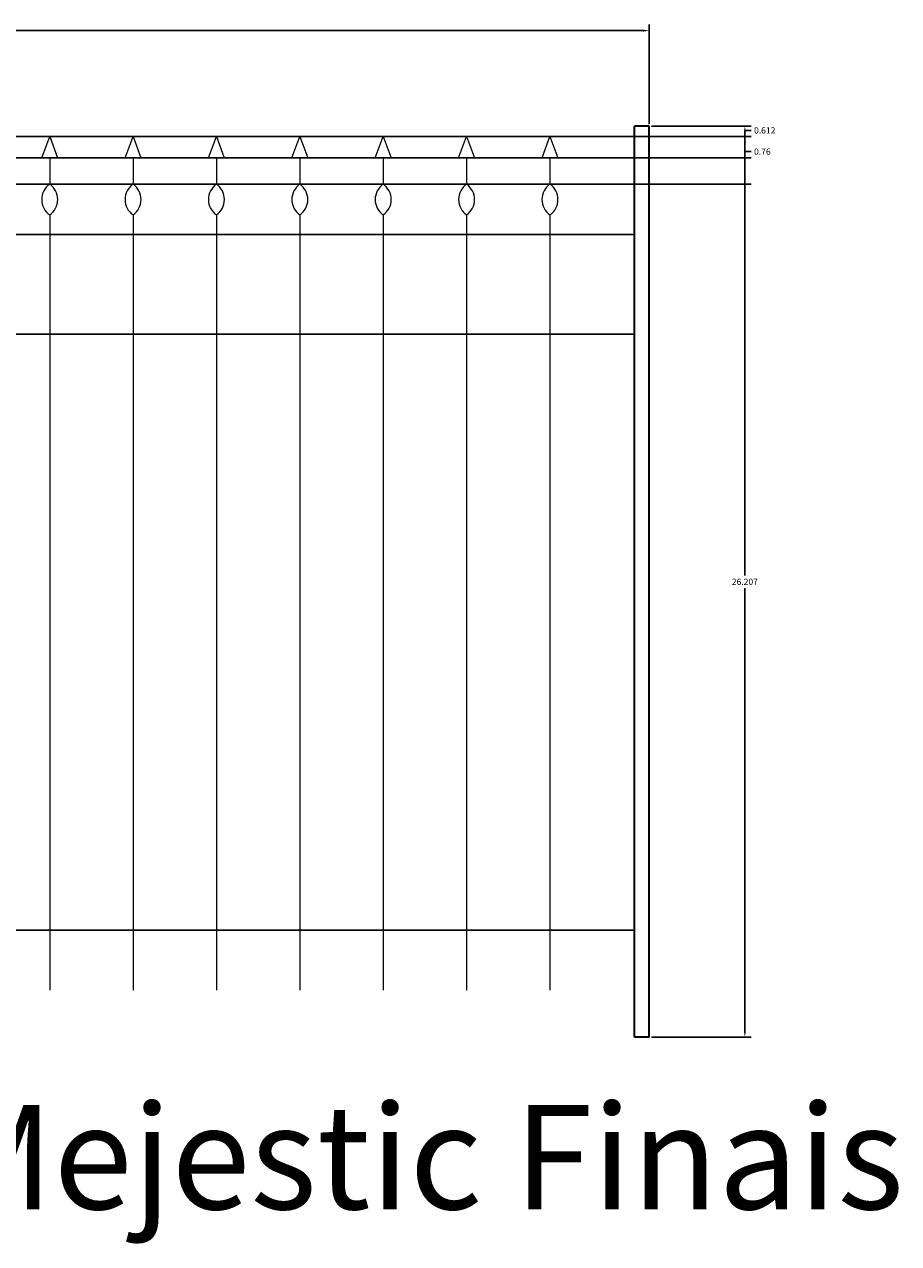
# Model space of a CAD drawing. Units: inches. Extents: x 756 to 915, y 488 to 695.
# Tile 25 of 25: x 888 to 913, y 660 to 695. Entities that reach past the tile are written whole.
import ezdxf

# ---------------------------------------------------------------- set-up
doc = ezdxf.new("R2010")
doc.units = ezdxf.units.IN
doc.header["$MEASUREMENT"] = 0
for name, color, linetype, lineweight in [('L-ANNO-TEXT', 7, 'Continuous', 25), ('L-FENC-PCKT', 7, 'Continuous', 18), ('L-FENC-POST', 7, 'Continuous', 35), ('L-FENC-RAIL', 7, 'Continuous', 25), ('M-DIMS', 2, 'Continuous', 18)]:
    doc.layers.add(name, color=color, linetype=linetype, lineweight=lineweight)
doc.styles.get("Standard").update_dxf_attribs({"font": 'arial.ttf'})
doc.dimstyles.get("Standard").update_dxf_attribs({"dimtxt": 0.18, "dimasz": 0.18, "dimexe": 0.18, "dimexo": 0.0625, "dimgap": 0.09, "dimtad": 0, "dimtih": 1, "dimtoh": 1, "dimdec": 0, "dimzin": 0, "dimdsep": 46, "dimlunit": 3, "dimtxsty": 'Standard', "dimcen": 0.09, "dimadec": 0, "dimazin": 0, "dimtfac": 1, "dimtdec": 0, "dimtofl": 0, "dimtmove": 0, "dimatfit": 3, "dimfxl": 1, "dimtolj": 1, "dimtzin": 0, "dimarcsym": 0})

# ---------------------------------------------------------------- blocks, each defined once
blk = doc.blocks.new('PICKET-MAJESTIC-EXTENDED')
for p, q in [((0.231, 23.946), (0.231, 23.188)), ((0.231, 22.305), (0.231, 0))]:
    blk.add_line(p, q)
blk.add_lwpolyline([(0.231, 23.946), (0.003, 23.946), (0.231, 24.558), (0.458, 23.946)], close=True)
blk.add_lwpolyline([(0.231, 22.305, 0.522719), (0.231, 23.188, 0.522719)], format="xyb", close=True)
blk = doc.blocks.new('FENCE-POST-RIGHT')
for p, q in [((0, 26.207), (0, 0)), ((0, 26.207), (0.427, 26.207)), ((0.427, 26.207), (0.427, 0)), ((0, 0), (0.427, 0))]:
    blk.add_line(p, q)
blk = doc.blocks.new('*D23')
at = {"layer": 'Defpoints', "color": 0, "transparency": 16777216}
for p in [(905.684, 694.703), (866.226, 691.953), (905.684, 691.953)]:
    blk.add_point(p, dxfattribs=at)
at = {"layer": 'M-DIMS', "color": 0, "lineweight": -2, "transparency": 16777216}
for p, q in [((866.226, 692.015), (866.226, 694.883)), ((905.684, 692.015), (905.684, 694.883)), ((866.406, 694.703), (885.561, 694.703)), ((905.504, 694.703), (886.348, 694.703))]:
    blk.add_line(p, q, dxfattribs=at)
at = {"layer": 'M-DIMS', "color": 0, "transparency": 16777216}
for points in [[(866.406, 694.733), (866.406, 694.673), (866.226, 694.703)], [(905.504, 694.733), (905.504, 694.673), (905.684, 694.703)]]:
    blk.add_solid(points, dxfattribs=at)
at = {"layer": 'M-DIMS', "color": 0, "transparency": 16777216, "insert": (885.955, 694.703), "char_height": 0.18, "attachment_point": 5}
blk.add_mtext('\\A1;39.46', dxfattribs=at)
blk = doc.blocks.new('*D24')
at = {"layer": 'Defpoints', "color": 0, "transparency": 16777216}
for p in [(905.684, 691.953), (908.434, 691.953), (905.684, 665.746)]:
    blk.add_point(p, dxfattribs=at)
at = {"layer": 'M-DIMS', "color": 0, "lineweight": -2, "transparency": 16777216}
for p, q in [((905.746, 691.953), (908.614, 691.953)), ((908.434, 691.773), (908.434, 679.031)), ((908.434, 665.926), (908.434, 678.668)), ((905.746, 665.746), (908.614, 665.746))]:
    blk.add_line(p, q, dxfattribs=at)
at = {"layer": 'M-DIMS', "color": 0, "transparency": 16777216}
for points in [[(908.404, 691.773), (908.464, 691.773), (908.434, 691.953)], [(908.404, 665.926), (908.464, 665.926), (908.434, 665.746)]]:
    blk.add_solid(points, dxfattribs=at)
at = {"layer": 'M-DIMS', "color": 0, "transparency": 16777216, "insert": (908.434, 678.849), "char_height": 0.18, "attachment_point": 5}
blk.add_mtext('\\A1;26.207', dxfattribs=at)
blk = doc.blocks.new('*D29')
at = {"layer": 'Defpoints', "color": 0, "transparency": 16777216}
for p in [(876.424, 691.654), (908.434, 691.654), (876.652, 691.042)]:
    blk.add_point(p, dxfattribs=at)
at = {"layer": 'M-DIMS', "color": 0, "lineweight": -2, "transparency": 16777216}
for p, q in [((876.487, 691.654), (908.614, 691.654)), ((908.434, 691.654), (908.434, 691.834)), ((908.434, 691.834), (908.614, 691.834)), ((908.434, 691.222), (908.434, 691.474)), ((876.714, 691.042), (908.614, 691.042))]:
    blk.add_line(p, q, dxfattribs=at)
at = {"layer": 'M-DIMS', "color": 0, "transparency": 16777216}
for points in [[(908.404, 691.474), (908.464, 691.474), (908.434, 691.654)], [(908.404, 691.222), (908.464, 691.222), (908.434, 691.042)]]:
    blk.add_solid(points, dxfattribs=at)
at = {"layer": 'M-DIMS', "color": 0, "transparency": 16777216, "insert": (909.006, 691.834), "char_height": 0.18, "attachment_point": 5}
blk.add_mtext('\\A1;0.612', dxfattribs=at)
blk = doc.blocks.new('*D30')
at = {"layer": 'Defpoints', "color": 0, "transparency": 16777216}
for p in [(876.652, 691.042), (908.434, 691.042), (876.424, 690.284)]:
    blk.add_point(p, dxfattribs=at)
at = {"layer": 'M-DIMS', "color": 0, "lineweight": -2, "transparency": 16777216}
for p, q in [((876.714, 691.042), (908.614, 691.042)), ((908.434, 691.042), (908.434, 691.222)), ((908.434, 691.222), (908.614, 691.222)), ((908.434, 690.464), (908.434, 690.862)), ((876.487, 690.284), (908.614, 690.284))]:
    blk.add_line(p, q, dxfattribs=at)
at = {"layer": 'M-DIMS', "color": 0, "transparency": 16777216}
for points in [[(908.404, 690.862), (908.464, 690.862), (908.434, 691.042)], [(908.404, 690.464), (908.464, 690.464), (908.434, 690.284)]]:
    blk.add_solid(points, dxfattribs=at)
at = {"layer": 'M-DIMS', "color": 0, "transparency": 16777216, "insert": (908.937, 691.222), "char_height": 0.18, "attachment_point": 5}
blk.add_mtext('\\A1;0.76', dxfattribs=at)

msp = doc.modelspace()

# ---------------------------------------------------------------- linework, layer by layer
at = {"layer": 'L-FENC-RAIL'}
for p, q in [((866.6522, 688.8379), (905.257, 688.8379)), ((866.6522, 685.9735), (905.257, 685.9735)), ((866.6522, 668.8277), (905.257, 668.8277))]:
    msp.add_line(p, q, dxfattribs=at)

# ---------------------------------------------------------------- block references
at = {"layer": 'L-FENC-PCKT'}
for p in [(888.1933, 667.096), (890.5932, 667.096), (892.9931, 667.096), (895.393, 667.096), (897.7929, 667.096), (900.1928, 667.096), (902.5928, 667.096)]:
    msp.add_blockref('PICKET-MAJESTIC-EXTENDED', p, dxfattribs=at)
at = {"layer": 'L-FENC-POST', "rotation": 180}
msp.add_blockref('FENCE-POST-RIGHT', (905.6838, 691.9529), dxfattribs=at)

# ---------------------------------------------------------------- texts
at = {"layer": 'L-ANNO-TEXT'}
msp.add_text('#111 With Mejestic Finais', height=3, dxfattribs=at).set_placement((865.5471, 660.7997))

# ---------------------------------------------------------------- dimensions: what is measured, and where the dimension line sits
at = {"layer": 'M-DIMS'}
dim = msp.add_linear_dim(base=(905.6837, 694.7029), p1=(866.2255, 691.9529), p2=(905.6837, 691.9529), dimstyle='Standard', override={"dimdec": 2, "dimlfac": 1, "dimrnd": 0, "dimzin": 0, "dimdsep": 46, "dimlunit": 2}, dxfattribs=at)
dim.commit()
dim.dimension.update_dxf_attribs({"geometry": '*D23', "text_midpoint": (885.9546, 694.7029)})
for base, p1, p2, override, picture, middle in [((908.4337, 691.6538), (876.6517, 691.0419), (876.4244, 691.6538), {"dimdec": 3, "dimlfac": 1, "dimrnd": 0, "dimzin": 0, "dimdsep": 46, "dimlunit": 2}, '*D29', (909.0065, 691.8338)), ((908.4337, 691.9529), (905.6837, 665.7461), (905.6837, 691.9529), {"dimdec": 3, "dimlfac": 1, "dimrnd": 0, "dimzin": 0, "dimdsep": 46, "dimlunit": 2}, '*D24', (908.4337, 678.8495)), ((908.4337, 691.0419), (876.4244, 690.2836), (876.6517, 691.0419), {"dimdec": 2, "dimlfac": 1, "dimrnd": 0, "dimzin": 0, "dimdsep": 46, "dimlunit": 2}, '*D30', (908.9374, 691.2219))]:
    dim = msp.add_linear_dim(base=base, p1=p1, p2=p2, angle=90, dimstyle='Standard', override=override, dxfattribs=at)
    dim.commit()
    dim.dimension.update_dxf_attribs({"geometry": picture, "text_midpoint": middle})

doc.saveas('drawing.dxf')
